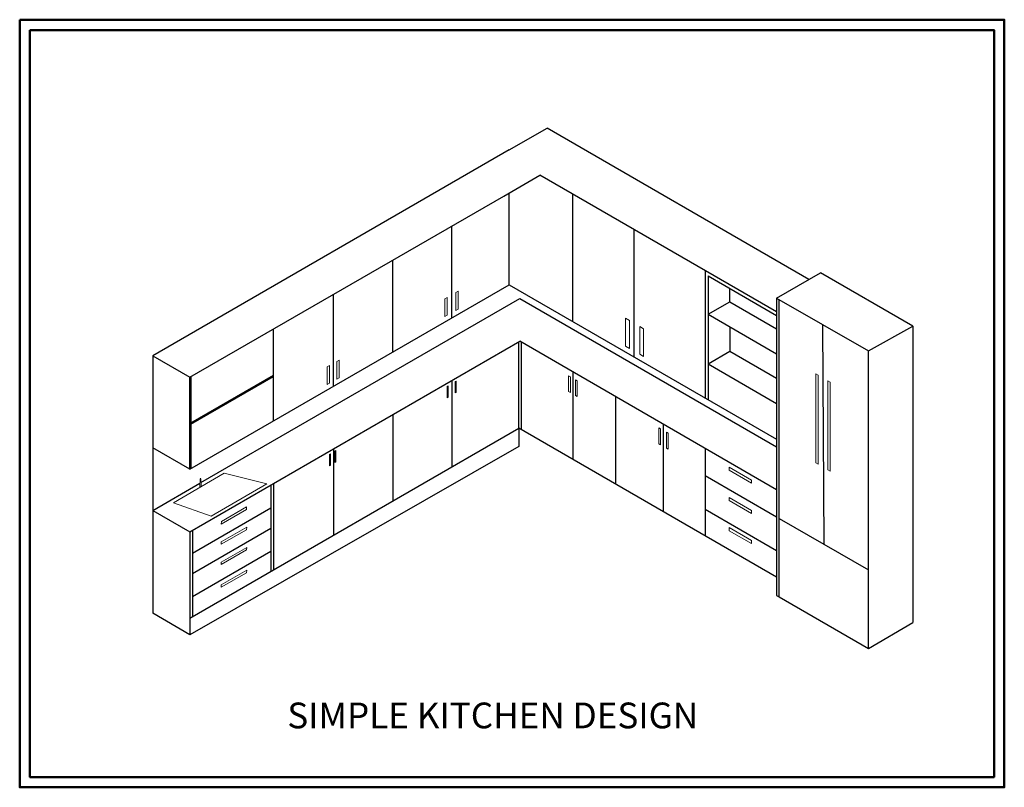
# Model space of a CAD drawing. Units: centimetres. Extents: x 97 to 8330, y -76 to 4066.
# Tile 1 of 2: x 97 to 1054, y -76 to 670. Entities that reach past the tile are written whole.
import ezdxf

# ---------------------------------------------------------------- set-up
doc = ezdxf.new("R2010")
doc.units = ezdxf.units.CM
doc.header["$MEASUREMENT"] = 0
for name, color, linetype, lineweight in [('A-ANNO-TEXT', 7, 'Continuous', 25), ('A-ANNO-TTLB', 7, 'Continuous', 50), ('A-FLOR-FIXT', 4, 'Continuous', 18), ('A-FURN', 7, 'Continuous', 25), ('A-FURN-HDWR', 8, 'Continuous', 18)]:
    doc.layers.add(name, color=color, linetype=linetype, lineweight=lineweight)
doc.styles.get("Standard").update_dxf_attribs({"font": 'arial.ttf'})

# ---------------------------------------------------------------- blocks, each defined once
blk = doc.blocks.new('PULL-DRAWER-A')
for p, q in [((24.68, 14.25), (0, 0)), ((0.11, 2.43), (24.68, 16.62)), ((24.68, 16.62), (24.68, 14.25)), ((0, 0), (0.11, 2.43))]:
    blk.add_line(p, q)
blk = doc.blocks.new('PULL-BASE-A')
for p, q in [((0, 10.99), (0.9, 11.51)), ((0, 10.99), (0, 0)), ((0.9, 0.52), (0.9, 11.51)), ((0, 0), (0.9, 0.52))]:
    blk.add_line(p, q)
blk = doc.blocks.new('PULL-BASE-B')
for p, q in [((0, 16.34), (0, 1.01)), ((0, 16.34), (1.74, 15.34)), ((1.74, 0), (1.74, 15.34)), ((0, 1.01), (1.74, 0))]:
    blk.add_line(p, q)
blk = doc.blocks.new('PULL-WALL-A')
for p, q in [((0, 17.22), (2.26, 18.53)), ((0, 17.22), (0, 0)), ((2.26, 1.3), (2.26, 18.53)), ((0, 0), (2.26, 1.3))]:
    blk.add_line(p, q)
blk = doc.blocks.new('PULL-DRAWER-B')
for p, q in [((0, 15.49), (21.75, 2.93)), ((0, 15.49), (0, 12.56)), ((21.75, 0), (0, 12.56)), ((21.75, 2.93), (21.75, 0))]:
    blk.add_line(p, q)
blk = doc.blocks.new('PULL-WALL-B')
for p, q in [((0, 29.15), (0, 2.14)), ((0, 29.15), (3.7, 27.01)), ((3.7, 0), (3.7, 27.01)), ((0, 2.14), (3.7, 0))]:
    blk.add_line(p, q)
blk = doc.blocks.new('PULL-TALL')
for p, q in [((0, 87.7), (0, 1.38)), ((0, 87.7), (2.39, 86.32)), ((2.39, 0), (2.39, 86.32)), ((0, 1.38), (2.39, 0))]:
    blk.add_line(p, q)

msp = doc.modelspace()

# ---------------------------------------------------------------- linework, layer by layer
at = {"layer": 'A-ANNO-TTLB'}
for points in [[(97.32, 669.85), (1054.27, 669.85), (1054.27, -75.66), (97.32, -75.66)], [(107.32, 659.85), (1044.27, 659.85), (1044.27, -65.66), (107.32, -65.66)]]:
    msp.add_lwpolyline(points, close=True, dxfattribs=at)
at = {"layer": 'A-FLOR-FIXT'}
for p, q in [((246.67, 200.74), (296.11, 229.29)), ((296.11, 229.29), (337.51, 218.98)), ((283.42, 187.75), (337.51, 218.98)), ((283.42, 187.75), (246.67, 200.74))]:
    msp.add_line(p, q, dxfattribs=at)
msp.add_ellipse((273.04, 215.97), major_axis=(0, 8.47), ratio=0.0665, start_param=4.750764, end_param=7.892356, dxfattribs=at)
at = {"layer": 'A-FURN'}
for p, q in [((573.2, 543.31), (609.82, 564.46)), ((864.25, 417.56), (609.82, 564.46)), ((573.2, 543.31), (226.79, 343.31)), ((567.77, 498.59), (602.89, 518.86)), ((833.01, 386), (602.89, 518.86)), ((262.81, 322.52), (567.77, 498.59)), ((573.2, 412.41), (573.2, 501.72)), ((634.94, 376.77), (634.94, 500.35)), ((517.45, 380.22), (517.45, 469.53)), ((694.46, 342.41), (694.46, 465.99)), ((459.94, 347.02), (459.94, 436.33)), ((763.48, 426.14), (763.48, 302.56)), ((833.01, 399.53), (875.58, 424.1)), ((965.43, 372.23), (875.58, 424.1)), ((262.81, 233.21), (573.2, 412.41)), ((573.2, 412.41), (833.01, 262.41)), ((766.44, 421.01), (833.01, 382.52)), ((766.44, 421.01), (766.44, 300.85)), ((402.24, 313.71), (402.24, 403.02)), ((787.58, 395.94), (787.58, 408.78)), ((273.53, 220.29), (583.26, 399.12)), ((583.26, 399.12), (833.01, 254.92)), ((766.44, 383.73), (787.58, 395.94)), ((787.58, 395.94), (833.01, 369.71)), ((833.01, 399.53), (833.01, 110.71)), ((833.01, 399.53), (922.13, 348.24)), ((835.52, 109.26), (835.52, 398.08)), ((766.44, 383.73), (833.01, 345.33)), ((877.57, 373.88), (878.82, 160.47)), ((344.03, 280.1), (344.03, 369.41)), ((787.58, 371.54), (787.58, 347.87)), ((922.13, 348.24), (965.43, 372.23)), ((965.43, 372.23), (965.43, 84.26)), ((262.81, 172.52), (583.26, 357.53)), ((582.57, 273.15), (582.57, 357.13)), ((833.01, 213.33), (583.26, 357.53)), ((585.11, 271.68), (585.11, 356.46)), ((766.44, 335.67), (787.58, 347.87)), ((787.58, 347.87), (833.01, 321.65)), ((922.13, 59.26), (922.13, 348.24)), ((226.79, 343.31), (226.79, 193.31)), ((226.79, 343.31), (262.81, 322.52)), ((766.44, 335.67), (833.01, 297.23)), ((634.94, 327.69), (634.94, 242.91)), ((262.81, 233.21), (262.81, 322.52)), ((263.5, 278.26), (344.03, 324.75)), ((263.5, 276.99), (344.03, 323.48)), ((263.5, 322.92), (263.5, 233.61)), ((517.45, 319.53), (517.45, 235.55)), ((676.34, 303.79), (676.34, 219.01)), ((459.94, 286.33), (459.94, 202.34)), ((262.81, 88.53), (582.57, 273.15)), ((833.01, 128.55), (582.57, 273.15)), ((582.57, 273.15), (582.57, 255.31)), ((722.83, 276.95), (722.83, 192.16)), ((262.81, 233.21), (226.79, 254.01)), ((582.57, 255.31), (262.81, 72.52)), ((402.24, 253.02), (402.24, 169.03)), ((763.48, 253.48), (763.48, 168.7)), ((763.48, 227.07), (833.01, 186.92)), ((226.79, 193.31), (272.54, 219.72)), ((341.55, 217.98), (341.55, 133.99)), ((344.03, 219.41), (344.03, 135.42)), ((226.79, 193.31), (262.81, 172.52)), ((226.79, 193.31), (226.79, 93.31)), ((265.31, 151.87), (341.55, 195.88)), ((763.48, 194.57), (833.01, 154.31)), ((835.52, 185.47), (922.13, 135.47)), ((262.81, 172.52), (262.81, 72.52)), ((265.33, 173.97), (265.25, 89.94)), ((265.29, 131.96), (341.55, 175.98)), ((265.27, 109.67), (341.55, 153.71)), ((833.01, 110.71), (835.52, 109.26)), ((835.52, 109.26), (922.13, 59.26)), ((262.81, 72.52), (226.79, 93.31)), ((922.13, 59.26), (965.43, 84.26))]:
    msp.add_line(p, q, dxfattribs=at)

# ---------------------------------------------------------------- block references
at = {"layer": 'A-FURN-HDWR'}
for name, p in [('PULL-WALL-A', (521.15, 387.56)), ('PULL-WALL-A', (510.64, 381.49)), ('PULL-WALL-B', (700.02, 342.73)), ('PULL-WALL-A', (405.4, 320.73)), ('PULL-WALL-A', (396.29, 315.47)), ('PULL-TALL', (871.02, 238.15)), ('PULL-BASE-B', (630.8, 307.69)), ('PULL-BASE-B', (637.51, 303.81)), ('PULL-TALL', (882.77, 231.37)), ('PULL-BASE-B', (718.53, 257.04)), ('PULL-BASE-B', (725.8, 252.84)), ('PULL-BASE-A', (403.76, 239.81)), ('PULL-DRAWER-B', (786.71, 219.77)), ('PULL-DRAWER-A', (293.22, 180.04))]:
    msp.add_blockref(name, p, dxfattribs=at)
for name, p, rotation in [('PULL-WALL-B', (689.96, 379.82), 180), ('PULL-BASE-A', (521.62, 318.85), 180), ('PULL-BASE-A', (513.65, 314.25), 180), ('PULL-BASE-A', (399.25, 248.19), 180), ('PULL-DRAWER-B', (808.46, 205.79), 180), ('PULL-DRAWER-A', (317.96, 176.99), 180.0165594904133), ('PULL-DRAWER-B', (808.46, 176.51), 180), ('PULL-DRAWER-A', (317.96, 157.29), 180.0165594904133), ('PULL-DRAWER-A', (317.96, 135.21), 180.0165594904133)]:
    msp.add_blockref(name, p, dxfattribs=dict(at, rotation=rotation))

# ---------------------------------------------------------------- texts
at = {"layer": 'A-ANNO-TEXT'}
msp.add_text('SIMPLE KITCHEN DESIGN', height=25, dxfattribs=at).set_placement((357.41, -18.37))

doc.saveas('drawing.dxf')
